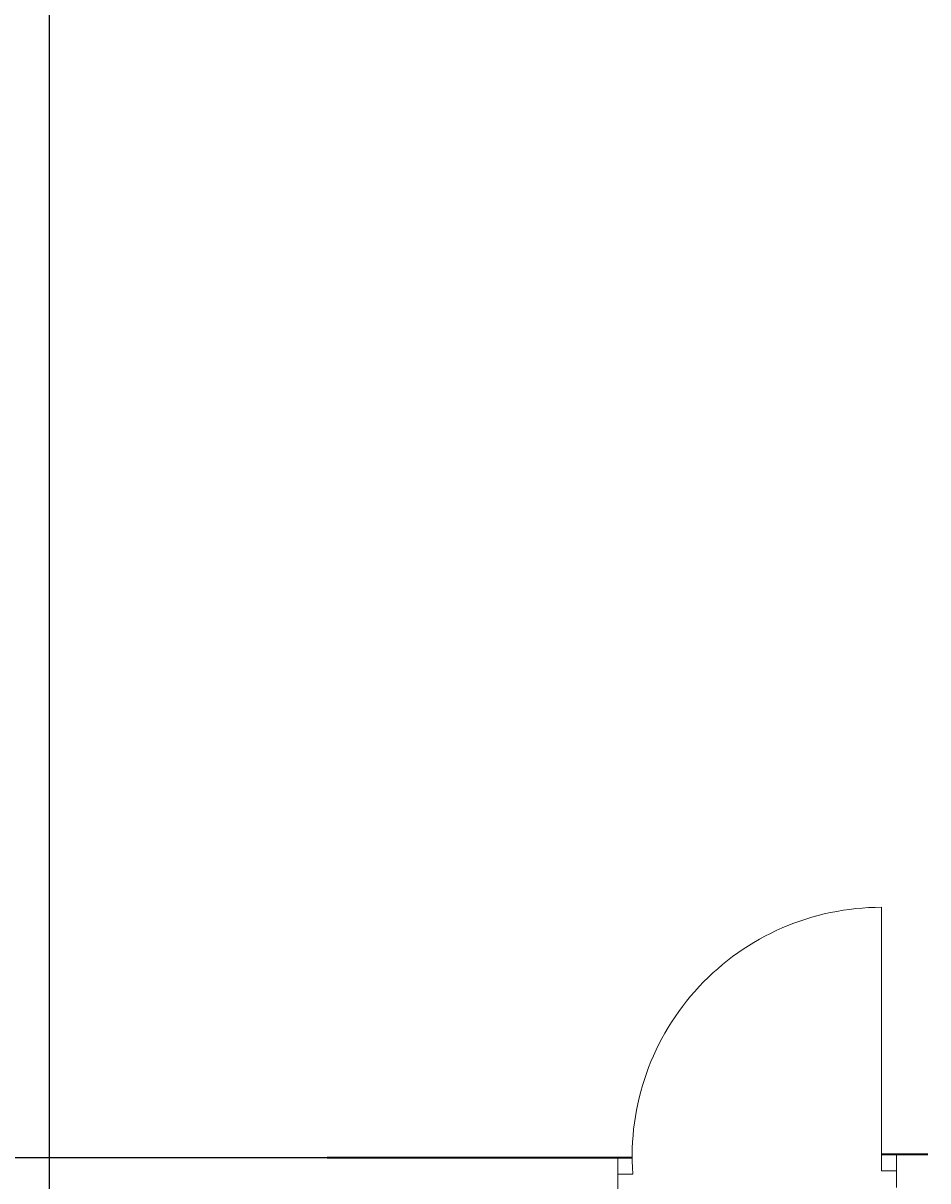
# Model space of a CAD drawing. Units: inches. Extents: x 1088 to 1703, y 668 to 1875.
# Tile 12 of 45: x 1314 to 1436, y 1416 to 1572. Entities that reach past the tile are written whole.
import ezdxf

# ---------------------------------------------------------------- set-up
doc = ezdxf.new("R2010")
doc.units = ezdxf.units.IN
for name, color, linetype, lineweight in [('A-ANNO-DIMS', 2, 'Continuous', 18), ('A-DOOR', 4, 'Continuous', 18), ('A-FLOR-EVTR', 5, 'Continuous', 25), ('A-WALL', 7, 'Continuous', 35)]:
    doc.layers.add(name, color=color, linetype=linetype, lineweight=lineweight)
doc.styles.get("Standard").update_dxf_attribs({"font": 'arial.ttf'})
doc.dimstyles.get("Standard").update_dxf_attribs({"dimtxt": 0.18, "dimasz": 0.18, "dimexe": 0.18, "dimexo": 0.0625, "dimgap": 0.09, "dimtad": 0, "dimtih": 1, "dimtoh": 1, "dimdec": 4, "dimzin": 0, "dimdsep": 46, "dimtxsty": 'Standard', "dimcen": 0.09, "dimadec": 0, "dimazin": 0, "dimtfac": 1, "dimtdec": 4, "dimtofl": 0, "dimtmove": 0, "dimatfit": 3, "dimfxl": 1, "dimtolj": 1, "dimtzin": 0, "dimarcsym": 0})

# ---------------------------------------------------------------- blocks, each defined once
blk = doc.blocks.new('*D38')
at = {"layer": 'A-ANNO-DIMS', "color": 0, "lineweight": -2, "transparency": 16777216}
for p, q in [((1317.34, 1736.94), (1317.34, 725.55)), ((1437.34, 1736.94), (1437.34, 725.55)), ((1317.52, 725.73), (1377.06, 725.73)), ((1437.16, 725.73), (1377.62, 725.73))]:
    blk.add_line(p, q, dxfattribs=at)
at = {"layer": 'A-ANNO-DIMS', "color": 0, "transparency": 16777216}
for points in [[(1317.52, 725.76), (1317.52, 725.7), (1317.34, 725.73)], [(1437.16, 725.76), (1437.16, 725.7), (1437.34, 725.73)]]:
    blk.add_solid(points, dxfattribs=at)
at = {"layer": 'Defpoints', "color": 0, "transparency": 16777216}
for p in [(1317.34, 1737.01), (1437.34, 1737.01), (1437.34, 725.73)]:
    blk.add_point(p, dxfattribs=at)
at = {"layer": 'A-ANNO-DIMS', "color": 0, "transparency": 16777216, "insert": (1377.34, 725.73), "char_height": 0.18, "attachment_point": 5}
blk.add_mtext('\\A1;120', dxfattribs=at)

msp = doc.modelspace()

# ---------------------------------------------------------------- linework, layer by layer
at = {"layer": 'A-DOOR'}
for p, q in [((1429.608, 1417.308), (1429.608, 1452.894)), ((1394.044, 1419.144), (1394.044, 1414.644)), ((1431.608, 1415.058), (1431.608, 1419.558)), ((1431.608, 1419.558), (1431.608, 1417.308)), ((1431.608, 1417.308), (1429.608, 1417.308)), ((1394.044, 1416.894), (1396.044, 1416.894))]:
    msp.add_line(p, q, dxfattribs=at)
msp.add_arc((1429.608, 1419.248), 33.646, 90, 184.01178, dxfattribs=at)
at = {"layer": 'A-FLOR-EVTR'}
for p in [(1294.845, 1419.144), (1354.845, 1419.144)]:
    msp.add_line(p, (1354.845, 1419.144), dxfattribs=at)
at = {"layer": 'A-WALL'}
for p, q in [((1354.845, 1419.144), (1394.044, 1419.144)), ((1394.044, 1419.144), (1395.962, 1419.144)), ((1429.608, 1419.558), (1435.845, 1419.558))]:
    msp.add_line(p, q, dxfattribs=at)

# ---------------------------------------------------------------- dimensions: what is measured, and where the dimension line sits
at = {"layer": 'A-ANNO-DIMS'}
dim = msp.add_linear_dim(base=(1437.345, 725.729), p1=(1317.345, 1737.007), p2=(1437.345, 1737.007), dimstyle='Standard', override={"dimdec": 0, "dimlfac": 1, "dimrnd": 0, "dimzin": 0, "dimdsep": 46, "dimlunit": 2}, dxfattribs=at)
dim.commit()
dim.dimension.update_dxf_attribs({"geometry": '*D38', "text_midpoint": (1377.345, 725.729)})

doc.saveas('drawing.dxf')
